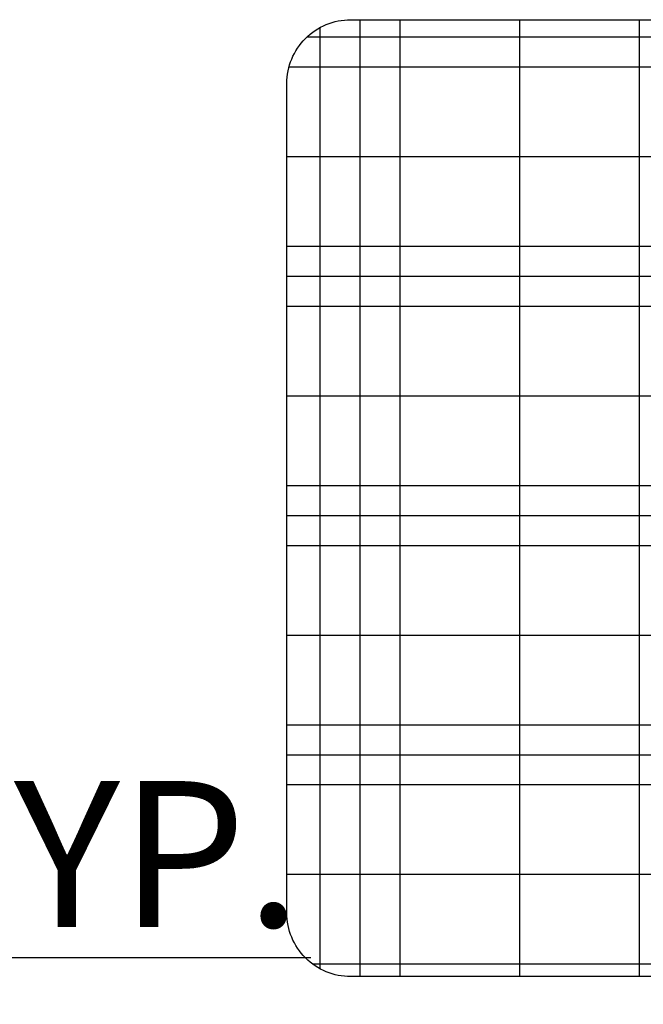
# Model space of a CAD drawing. Units: inches. Extents: x 3064 to 19385, y 846 to 15425.
# Tile 95 of 108: x 7574 to 7612, y 1032 to 1093. Entities that reach past the tile are written whole.
import ezdxf

# ---------------------------------------------------------------- set-up
doc = ezdxf.new("R2010")
doc.units = ezdxf.units.IN
doc.layers.add('A-ANNO-DIMS', color=2, linetype='Continuous', lineweight=18)
doc.layers.add('A-FLOR-FIXT', color=9, linetype='Continuous', lineweight=18)
doc.layers.add('BLOCK', color=6, linetype='Continuous')
doc.styles.get("Standard").update_dxf_attribs({"font": 'arial.ttf'})
doc.dimstyles.new('ISO-25', dxfattribs={"dimtxt": 9, "dimasz": 2.5, "dimexe": 1.25, "dimexo": 0.625, "dimtad": 1, "dimdec": 1, "dimlunit": 3, "dimtxsty": 'Standard', "dimcen": 2.5, "dimadec": 0, "dimazin": 0, "dimtfac": 1, "dimtdec": 1, "dimtmove": 0, "dimatfit": 3, "dimfxl": 1, "dimarcsym": 0})

# ---------------------------------------------------------------- blocks, each defined once
blk = doc.blocks.new('*X5')
at = {"color": 0}
for p, q in [((276.598, 451.25), (280.51, 451.25)), ((275.455, 450.625), (280.51, 450.625)), ((274.411, 450), (280.51, 450)), ((265.51, 448.125), (267.634, 448.125)), ((271.723, 448.125), (280.51, 448.125)), ((265.51, 446.25), (268.465, 446.25)), ((269.519, 446.25), (280.51, 446.25)), ((265.51, 445.625), (268.531, 445.625)), ((268.866, 445.625), (280.51, 445.625)), ((265.51, 445), (280.51, 445)), ((265.51, 443.125), (280.51, 443.125)), ((265.51, 441.25), (280.51, 441.25)), ((265.51, 440.625), (280.51, 440.625)), ((265.634, 440), (280.386, 440))]:
    blk.add_line(p, q, dxfattribs=at)
blk = doc.blocks.new('*X6')
at = {"color": 0}
for p, q in [((280.312, 439.886), (280.312, 452.896)), ((278.906, 439.482), (278.906, 452.338)), ((277.5, 439.482), (277.5, 451.702)), ((277.031, 439.482), (277.031, 451.471)), ((276.562, 439.482), (276.562, 451.231)), ((275.156, 439.482), (275.156, 450.451)), ((265.781, 439.797), (265.781, 449.511)), ((273.75, 439.482), (273.75, 449.576)), ((266.25, 439.517), (266.25, 449.296)), ((273.281, 439.482), (273.281, 449.261)), ((272.812, 439.482), (272.812, 448.934)), ((267.656, 439.482), (267.656, 448.095)), ((271.406, 439.482), (271.406, 447.876)), ((270, 439.482), (270, 446.689)), ((269.531, 439.482), (269.531, 446.262)), ((269.062, 439.482), (269.062, 445.817))]:
    blk.add_line(p, q, dxfattribs=at)
blk = doc.blocks.new('A$C52E67D0D')
at = {"layer": 'BLOCK'}
blk.add_lwpolyline([(1901, 0), (601, 0, -0.414214), (501, 100), (501, 1700, -0.414214), (601, 1800), (1901, 1800, -0.414214), (2001, 1700), (2001, 100, -0.414214)], format="xyb", close=True, dxfattribs=at)
at = {"layer": 'BLOCK', "xscale": 100, "yscale": 100, "zscale": 100}
for name in ['*X6', '*X5']:
    blk.add_blockref(name, (-26050, -43948.2), dxfattribs=at)
blk = doc.blocks.new('*D432')
at = {"layer": 'A-ANNO-DIMS', "color": 0, "lineweight": -2, "transparency": 16777216}
for p, q in [((7527.746, 1044.715), (7527.746, 1033.74)), ((7530.746, 1044.715), (7530.746, 1033.74)), ((7525.246, 1034.99), (7522.746, 1034.99)), ((7527.746, 1034.99), (7530.746, 1034.99)), ((7533.246, 1034.99), (7591.856, 1034.99))]:
    blk.add_line(p, q, dxfattribs=at)
at = {"layer": 'A-ANNO-DIMS', "color": 0, "transparency": 16777216}
for points in [[(7525.246, 1035.407), (7525.246, 1034.573), (7527.746, 1034.99)], [(7533.246, 1035.407), (7533.246, 1034.573), (7530.746, 1034.99)]]:
    blk.add_solid(points, dxfattribs=at)
at = {"layer": 'Defpoints', "color": 0, "transparency": 16777216}
for p in [(7527.746, 1045.34), (7530.746, 1045.34), (7530.746, 1034.99)]:
    blk.add_point(p, dxfattribs=at)
at = {"layer": 'A-ANNO-DIMS', "color": 0, "transparency": 16777216, "insert": (7563.801, 1040.213), "char_height": 9, "attachment_point": 5}
blk.add_mtext('0\'-3" TYP.', dxfattribs=at)

msp = doc.modelspace()

# ---------------------------------------------------------------- block references
at = {"layer": 'A-FLOR-FIXT', "xscale": 0.039370099999992, "yscale": 0.039370099999992, "zscale": 0.039370099999992, "rotation": 270}
msp.add_blockref('A$C52E67D0D', (7590.38, 1112.592), dxfattribs=at)

# ---------------------------------------------------------------- dimensions: what is measured, and where the dimension line sits
at = {"layer": 'A-ANNO-DIMS'}
dim = msp.add_linear_dim(base=(7530.746, 1034.99), p1=(7527.746, 1045.34), p2=(7530.746, 1045.34), text='<> TYP.', dimstyle='ISO-25', override={"dimdec": 1, "dimrnd": 0, "dimzin": 1, "dimlunit": 4, "dimfrac": 2}, dxfattribs=at)
dim.commit()
dim.dimension.update_dxf_attribs({"geometry": '*D432', "text_midpoint": (7563.801, 1040.213)})

doc.saveas('drawing.dxf')
